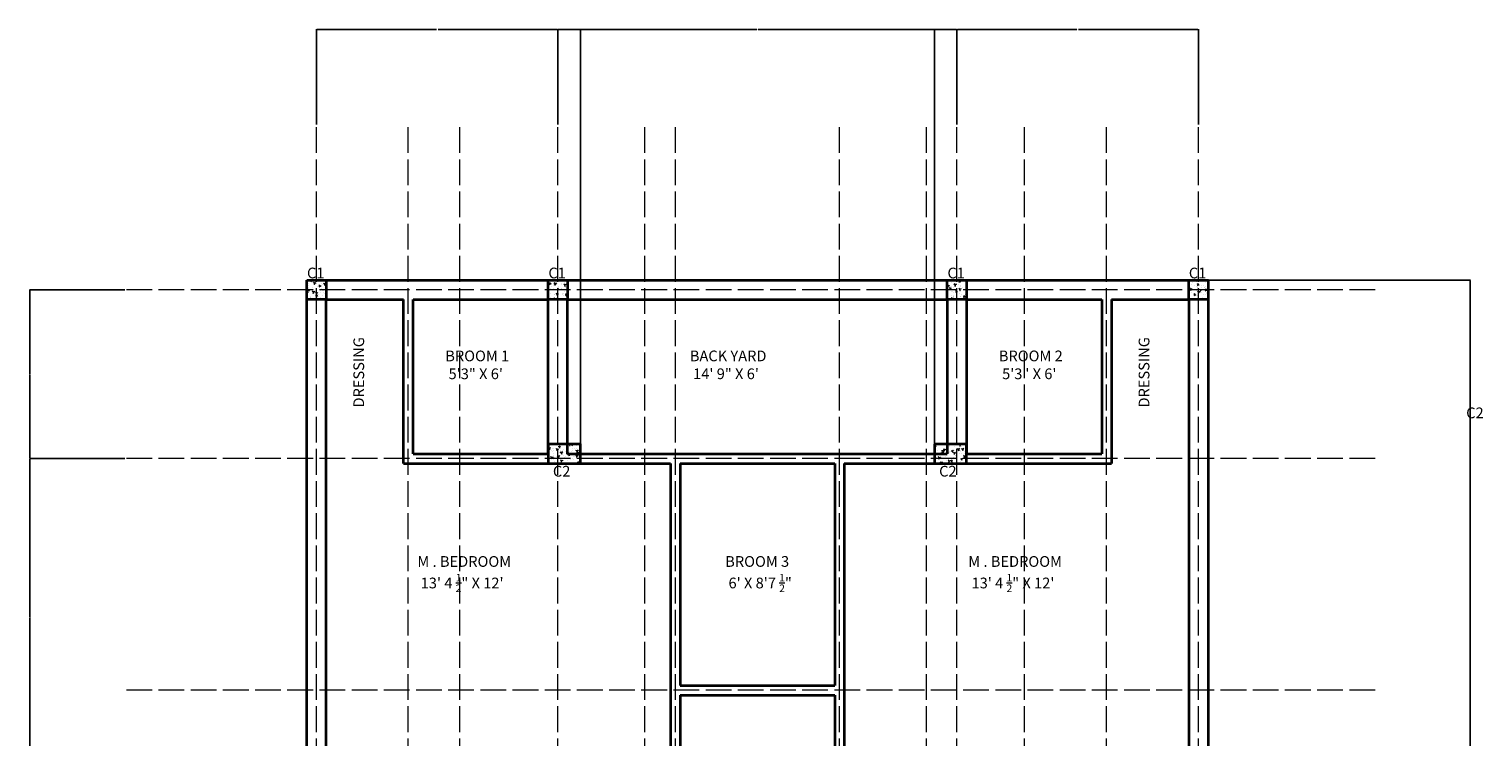
# Model space of a CAD drawing. Units: inches. Extents: x 1159 to 4240, y 1112 to 2085.
# Tile 12 of 13: x 2561 to 3239, y 1755 to 2085. Entities that reach past the tile are written whole.
import ezdxf

# ---------------------------------------------------------------- set-up
doc = ezdxf.new("R2010")
doc.units = ezdxf.units.IN
doc.linetypes.add('ACAD_ISO02W100', pattern=[15, 12, -3])
for name, color, linetype, lineweight in [('A-ANNO-DIMS', 2, 'Continuous', 18), ('A-AREA-IDEN', 30, 'Continuous', 18), ('A-GRID', 8, 'ACAD_ISO02W100', 13), ('COLUMN', 120, 'Continuous', 35), ('column no', 210, 'Continuous', 18), ('WALL', 7, 'Continuous', 35)]:
    doc.layers.add(name, color=color, linetype=linetype, lineweight=lineweight)
doc.styles.get("Standard").update_dxf_attribs({"font": 'arial.ttf'})
doc.dimstyles.get("Standard").update_dxf_attribs({"dimtxt": 0.18, "dimasz": 0.18, "dimexe": 0.18, "dimexo": 0.0625, "dimgap": 0.09, "dimtad": 0, "dimtih": 1, "dimtoh": 1, "dimdec": 4, "dimzin": 0, "dimdsep": 46, "dimtxsty": 'Standard', "dimcen": 0.09, "dimadec": 0, "dimazin": 0, "dimtfac": 1, "dimtdec": 4, "dimtofl": 0, "dimtmove": 0, "dimatfit": 3, "dimfxl": 1, "dimtolj": 1, "dimtzin": 0, "dimarcsym": 0})

# ---------------------------------------------------------------- blocks, each defined once
blk = doc.blocks.new('column')
at = {"layer": 'COLUMN'}
h = blk.add_hatch(dxfattribs=at)
h.set_pattern_fill('AR-CONC', color=256, scale=0.025)
h.set_pattern_definition([(50, (-3308.5408, -1592.3894), (4.5546167, -0.398477), [0.47625, -5.23875]), (355, (-3308.541, -1592.3894), (-0.8810855, 4.776421), [0.381, -4.1910146]), (100.45144, (-3308.1612, -1592.4226), (3.673531, 4.377944), [0.40475, -4.452256]), (46.1842, (-3308.541, -1591.1194), (6.776976, -1.051058), [0.714375, -7.858125]), (96.63556, (-3307.976, -1591.207), (5.935103, 6.185653), [0.607126, -6.67839]), (351.18415, (-3308.541, -1591.1194), (5.935103, 6.185653), [0.571499, -6.286493]), (21, (-3307.9058, -1591.437), (3.7903598, -2.55663), [0.47625, -5.23875]), (326, (-3307.906, -1591.437), (1.545051, 4.604699), [0.381, -4.191]), (71.45144, (-3307.59, -1591.65), (5.3354105, 2.048069), [0.40475, -4.4522484]), (37.5, (-3308.5408, -1592.3894), (0.0772151, 2.113876), [0, -4.1402, 0, -4.2545, 0, -4.206875]), (7.5, (-3308.5408, -1592.3894), (1.6704916, 2.5045144), [0, -2.4257, 0, -4.04495, 0, -1.603375]), (327.5, (-3309.9568, -1592.3894), (3.3897649, -0.1432186), [0, -1.5875, 0, -4.953, 0, -6.57225]), (317.5, (-3310.5918, -1592.3894), (3.7032295, 0.6356623), [0, -2.06375, 0, -3.2893, 0, -4.66725])])
h.paths.add_polyline_path([(0, 9), (0, 0), (9, 0), (9, 9)])
blk.add_lwpolyline([(0, 9), (9, 9), (9, 0), (0, 0)], close=True, dxfattribs=at)
blk = doc.blocks.new('colum 1')
at = {"layer": 'COLUMN'}
h = blk.add_hatch(dxfattribs=at)
h.set_pattern_fill('AR-CONC', color=256, scale=0.025)
h.set_pattern_definition([(50, (-3344.692, -1599.4877), (4.5546167, -0.398477), [0.47625, -5.23875]), (355, (-3344.692, -1599.4877), (-0.8810855, 4.776421), [0.381, -4.1910146]), (100.45144, (-3344.3125, -1599.521), (3.673531, 4.377944), [0.40475, -4.452256]), (46.1842, (-3344.692, -1598.218), (6.776976, -1.051058), [0.714375, -7.858125]), (96.63556, (-3344.127, -1598.305), (5.935103, 6.185653), [0.607126, -6.67839]), (351.18415, (-3344.692, -1598.218), (5.935103, 6.185653), [0.571499, -6.286493]), (21, (-3344.057, -1598.5352), (3.7903598, -2.55663), [0.47625, -5.23875]), (326, (-3344.057, -1598.5352), (1.545051, 4.604699), [0.381, -4.191]), (71.45144, (-3343.741, -1598.7483), (5.3354105, 2.048069), [0.40475, -4.4522484]), (37.5, (-3344.692, -1599.4877), (0.0772151, 2.113876), [0, -4.1402, 0, -4.2545, 0, -4.206875]), (7.5, (-3344.692, -1599.4877), (1.6704916, 2.5045144), [0, -2.4257, 0, -4.04495, 0, -1.603375]), (327.5, (-3346.1081, -1599.4877), (3.3897649, -0.1432186), [0, -1.5875, 0, -4.953, 0, -6.57225]), (317.5, (-3346.743, -1599.4877), (3.7032295, 0.6356623), [0, -2.06375, 0, -3.2893, 0, -4.66725])])
h.paths.add_polyline_path([(9, 15), (0, 15), (0, 0), (9, 0)])
blk.add_lwpolyline([(0, 0), (9, 0), (9, 15), (0, 15)], close=True, dxfattribs=at)
blk = doc.blocks.new('HOUSE-35x60-WALL-LAYOUT')
for p, q in [((0, 0), (0, 720)), ((0, 720), (420, 720)), ((420, 720), (420, 297)), ((9, 711), (45, 711)), ((9, 634.5), (9, 711)), ((45, 634.5), (45, 711)), ((49.5, 639), (49.5, 711)), ((49.5, 711), (112.5, 711)), ((112.5, 639), (112.5, 711)), ((121.5, 639), (121.5, 711)), ((121.5, 711), (298.5, 711)), ((298.5, 711), (298.5, 639)), ((307.5, 711), (307.5, 639)), ((307.5, 711), (370.5, 711)), ((370.5, 711), (370.5, 639)), ((375, 711), (375, 634.5)), ((375, 711), (411, 711)), ((411, 711), (411, 634.5)), ((49.5, 639), (112.5, 639)), ((121.5, 639), (298.5, 639)), ((307.5, 639), (370.5, 639)), ((9, 490.5), (9, 634.5)), ((45, 634.5), (169.5, 634.5)), ((169.5, 634.5), (169.5, 490.5)), ((174, 634.5), (174, 531)), ((174, 634.5), (246, 634.5)), ((246, 634.5), (246, 531)), ((250.5, 634.5), (250.5, 490.5)), ((250.5, 634.5), (375, 634.5)), ((411, 634.5), (411, 490.5)), ((174, 531), (246, 531)), ((174, 526.5), (246, 526.5)), ((174, 526.5), (174, 486)), ((246, 526.5), (246, 486)), ((9, 490.5), (169.5, 490.5)), ((250.5, 490.5), (411, 490.5)), ((9, 486), (174, 486)), ((9, 306), (9, 486)), ((246, 486), (286.5, 486)), ((286.5, 486), (286.5, 421.5)), ((291, 486), (291, 426)), ((291, 486), (411, 486)), ((411, 486), (411, 426)), ((291, 421.5), (286.5, 421.5)), ((291, 426), (411, 426)), ((291, 421.5), (411, 421.5)), ((411, 421.5), (411, 306)), ((291, 361.5), (286.5, 361.5)), ((286.5, 361.5), (286.5, 297)), ((291, 361.5), (291, 306)), ((9, 306), (157.5, 306)), ((157.5, 190.5), (157.5, 306)), ((291, 306), (411, 306)), ((9, 297), (153, 297)), ((9, 190.5), (9, 297)), ((153, 190.5), (153, 297)), ((286.5, 297), (420, 297)), ((330, 297), (330, 123)), ((339, 297), (339, 114)), ((153, 190.5), (9, 190.5)), ((157.5, 123), (157.5, 190.5)), ((9, 66), (9, 186)), ((153, 186), (9, 186)), ((153, 66), (153, 186)), ((330, 123), (157.5, 123)), ((162, 57), (162, 114)), ((339, 114), (162, 114)), ((153, 66), (9, 66)), ((9, 9), (9, 57)), ((69, 57), (9, 57)), ((69, 9), (69, 57)), ((162, 57), (73.5, 57)), ((73.5, 0), (73.5, 57)), ((69, 9), (9, 9)), ((0, 0), (73.5, 0))]:
    blk.add_line(p, q)
blk = doc.blocks.new('HOUSE-35x60-SETTING-OUT-GRID')
for p, q in [((89.32, 0), (89.32, 883.25)), ((132.07, 0), (132.07, 883.25)), ((156.07, 0), (156.07, 883.25)), ((201.82, 0), (201.82, 883.25)), ((242.32, 0), (242.32, 883.25)), ((256.57, 0), (256.57, 883.25)), ((333.07, 0), (333.07, 883.25)), ((373.57, 0), (373.57, 883.25)), ((387.82, 0), (387.82, 883.25)), ((419.32, 0), (419.32, 883.25)), ((457.57, 0), (457.57, 883.25)), ((500.32, 0), (500.32, 883.25)), ((582.7, 806.25), (0, 806.25)), ((582.7, 727.5), (0, 727.5)), ((582.7, 619.5), (0, 619.5)), ((582.7, 579), (0, 579)), ((582.7, 514.5), (0, 514.5)), ((582.7, 392.25), (0, 392.25)), ((582.7, 279), (0, 279)), ((582.7, 209.25), (0, 209.25)), ((582.7, 152.25), (0, 152.25)), ((582.7, 95.25), (0, 95.25))]:
    blk.add_line(p, q)
blk = doc.blocks.new('*D25')
at = {"layer": 'A-ANNO-DIMS', "color": 0, "lineweight": -2, "transparency": 16777216}
for p, q in [((3110.55, 1967.7), (3232.9, 1967.7)), ((3232.72, 1967.52), (3232.72, 1607.88)), ((3232.72, 1247.88), (3232.72, 1607.52)), ((3110.55, 1247.7), (3232.9, 1247.7))]:
    blk.add_line(p, q, dxfattribs=at)
at = {"layer": 'A-ANNO-DIMS', "color": 0, "lineweight": 100, "transparency": 16777216}
for points in [[(3232.69, 1967.52), (3232.75, 1967.52), (3232.72, 1967.7)], [(3232.69, 1247.88), (3232.75, 1247.88), (3232.72, 1247.7)]]:
    blk.add_solid(points, dxfattribs=at)
at = {"layer": 'Defpoints', "color": 0, "lineweight": 100, "transparency": 16777216}
for p in [(3110.48, 1967.7), (3232.72, 1967.7), (3110.48, 1247.7)]:
    blk.add_point(p, dxfattribs=at)
at = {"layer": 'A-ANNO-DIMS', "color": 0, "transparency": 16777216, "insert": (3232.72, 1607.7), "char_height": 0.18, "attachment_point": 5}
blk.add_mtext('\\A1;720', dxfattribs=at)
blk = doc.blocks.new('*D46')
at = {"layer": 'A-ANNO-DIMS', "color": 0, "lineweight": -2, "transparency": 16777216}
for p, q in [((2694.98, 2040.27), (2694.98, 2084.73)), ((2695.16, 2084.55), (2750.85, 2084.55)), ((2807.3, 2084.55), (2751.62, 2084.55)), ((2807.48, 2040.27), (2807.48, 2084.73))]:
    blk.add_line(p, q, dxfattribs=at)
at = {"layer": 'A-ANNO-DIMS', "color": 0, "lineweight": 100, "transparency": 16777216}
for points in [[(2695.16, 2084.58), (2695.16, 2084.52), (2694.98, 2084.55)], [(2807.3, 2084.58), (2807.3, 2084.52), (2807.48, 2084.55)]]:
    blk.add_solid(points, dxfattribs=at)
at = {"layer": 'Defpoints', "color": 0, "lineweight": 100, "transparency": 16777216}
for p in [(2807.48, 2084.55), (2694.98, 2040.2), (2807.48, 2040.2)]:
    blk.add_point(p, dxfattribs=at)
at = {"layer": 'A-ANNO-DIMS', "color": 0, "transparency": 16777216, "insert": (2751.23, 2084.55), "char_height": 0.18, "attachment_point": 5}
blk.add_mtext('\\A1;112.5', dxfattribs=at)
blk = doc.blocks.new('*D47')
at = {"layer": 'A-ANNO-DIMS', "color": 0, "lineweight": -2, "transparency": 16777216}
for p, q in [((2807.48, 2040.27), (2807.48, 2084.73)), ((2807.66, 2084.55), (2900.2, 2084.55)), ((2993.3, 2084.55), (2900.76, 2084.55)), ((2993.48, 2040.27), (2993.48, 2084.73))]:
    blk.add_line(p, q, dxfattribs=at)
at = {"layer": 'A-ANNO-DIMS', "color": 0, "lineweight": 100, "transparency": 16777216}
for points in [[(2807.66, 2084.58), (2807.66, 2084.52), (2807.48, 2084.55)], [(2993.3, 2084.58), (2993.3, 2084.52), (2993.48, 2084.55)]]:
    blk.add_solid(points, dxfattribs=at)
at = {"layer": 'Defpoints', "color": 0, "lineweight": 100, "transparency": 16777216}
for p in [(2993.48, 2084.55), (2807.48, 2040.2), (2993.48, 2040.2)]:
    blk.add_point(p, dxfattribs=at)
at = {"layer": 'A-ANNO-DIMS', "color": 0, "transparency": 16777216, "insert": (2900.48, 2084.55), "char_height": 0.18, "attachment_point": 5}
blk.add_mtext('\\A1;186', dxfattribs=at)
blk = doc.blocks.new('*D48')
at = {"layer": 'A-ANNO-DIMS', "color": 0, "lineweight": -2, "transparency": 16777216}
for p, q in [((2993.48, 2040.27), (2993.48, 2084.73)), ((2993.66, 2084.55), (3049.35, 2084.55)), ((3105.8, 2084.55), (3050.12, 2084.55)), ((3105.98, 2040.27), (3105.98, 2084.73))]:
    blk.add_line(p, q, dxfattribs=at)
at = {"layer": 'A-ANNO-DIMS', "color": 0, "lineweight": 100, "transparency": 16777216}
for points in [[(2993.66, 2084.58), (2993.66, 2084.52), (2993.48, 2084.55)], [(3105.8, 2084.58), (3105.8, 2084.52), (3105.98, 2084.55)]]:
    blk.add_solid(points, dxfattribs=at)
at = {"layer": 'Defpoints', "color": 0, "lineweight": 100, "transparency": 16777216}
for p in [(3105.98, 2084.55), (2993.48, 2040.2), (3105.98, 2040.2)]:
    blk.add_point(p, dxfattribs=at)
at = {"layer": 'A-ANNO-DIMS', "color": 0, "transparency": 16777216, "insert": (3049.73, 2084.55), "char_height": 0.18, "attachment_point": 5}
blk.add_mtext('\\A1;112.5', dxfattribs=at)
blk = doc.blocks.new('*D50')
at = {"layer": 'A-ANNO-DIMS', "color": 0, "lineweight": -2, "transparency": 16777216}
for p, q in [((2605.61, 1884.45), (2561.14, 1884.45)), ((2561.32, 1884.27), (2561.32, 1810.38)), ((2561.32, 1736.13), (2561.32, 1810.02)), ((2605.61, 1735.95), (2561.14, 1735.95))]:
    blk.add_line(p, q, dxfattribs=at)
at = {"layer": 'A-ANNO-DIMS', "color": 0, "lineweight": 100, "transparency": 16777216}
for points in [[(2561.29, 1884.27), (2561.35, 1884.27), (2561.32, 1884.45)], [(2561.29, 1736.13), (2561.35, 1736.13), (2561.32, 1735.95)]]:
    blk.add_solid(points, dxfattribs=at)
at = {"layer": 'Defpoints', "color": 0, "lineweight": 100, "transparency": 16777216}
for p in [(2561.32, 1884.45), (2605.67, 1884.45), (2605.67, 1735.95)]:
    blk.add_point(p, dxfattribs=at)
at = {"layer": 'A-ANNO-DIMS', "color": 0, "transparency": 16777216, "insert": (2561.32, 1810.2), "char_height": 0.18, "attachment_point": 5}
blk.add_mtext('\\A1;148.5', dxfattribs=at)
blk = doc.blocks.new('*D51')
at = {"layer": 'A-ANNO-DIMS', "color": 0, "lineweight": -2, "transparency": 16777216}
for p, q in [((2605.61, 1963.2), (2561.14, 1963.2)), ((2561.32, 1963.02), (2561.32, 1924.01)), ((2561.32, 1884.63), (2561.32, 1923.65)), ((2605.61, 1884.45), (2561.14, 1884.45))]:
    blk.add_line(p, q, dxfattribs=at)
at = {"layer": 'A-ANNO-DIMS', "color": 0, "lineweight": 100, "transparency": 16777216}
for points in [[(2561.29, 1963.02), (2561.35, 1963.02), (2561.32, 1963.2)], [(2561.29, 1884.63), (2561.35, 1884.63), (2561.32, 1884.45)]]:
    blk.add_solid(points, dxfattribs=at)
at = {"layer": 'Defpoints', "color": 0, "lineweight": 100, "transparency": 16777216}
for p in [(2561.32, 1963.2), (2605.67, 1963.2), (2605.67, 1884.45)]:
    blk.add_point(p, dxfattribs=at)
at = {"layer": 'A-ANNO-DIMS', "color": 0, "transparency": 16777216, "insert": (2561.32, 1923.83), "char_height": 0.18, "attachment_point": 5}
blk.add_mtext('\\A1;78.75', dxfattribs=at)
blk = doc.blocks.new('*D52')
at = {"layer": 'A-ANNO-DIMS', "color": 0, "lineweight": -2, "transparency": 16777216}
for p, q in [((2817.98, 1891.26), (2817.98, 2084.73)), ((2818.16, 2084.55), (2900.2, 2084.55)), ((2982.8, 2084.55), (2900.76, 2084.55)), ((2982.98, 1891.26), (2982.98, 2084.73))]:
    blk.add_line(p, q, dxfattribs=at)
at = {"layer": 'A-ANNO-DIMS', "color": 0, "lineweight": 100, "transparency": 16777216}
for points in [[(2818.16, 2084.58), (2818.16, 2084.52), (2817.98, 2084.55)], [(2982.8, 2084.58), (2982.8, 2084.52), (2982.98, 2084.55)]]:
    blk.add_solid(points, dxfattribs=at)
at = {"layer": 'Defpoints', "color": 0, "lineweight": 100, "transparency": 16777216}
for p in [(2982.98, 2084.55), (2817.98, 1891.2), (2982.98, 1891.2)]:
    blk.add_point(p, dxfattribs=at)
at = {"layer": 'A-ANNO-DIMS', "color": 0, "transparency": 16777216, "insert": (2900.48, 2084.55), "char_height": 0.18, "attachment_point": 5}
blk.add_mtext('\\A1;165', dxfattribs=at)

msp = doc.modelspace()

# ---------------------------------------------------------------- block references
at = {"layer": 'A-GRID'}
msp.add_blockref('HOUSE-35x60-SETTING-OUT-GRID', (2605.668, 1156.954), dxfattribs=at)
at = {"layer": 'COLUMN'}
for p in [(2690.484, 1958.702), (2802.984, 1958.702), (2988.984, 1958.702), (3101.484, 1958.702)]:
    msp.add_blockref('column', p, dxfattribs=at)
at = {"layer": 'COLUMN', "rotation": 270}
for p in [(2802.984, 1891.202), (2982.984, 1891.202)]:
    msp.add_blockref('colum 1', p, dxfattribs=at)
at = {"layer": 'WALL'}
msp.add_blockref('HOUSE-35x60-WALL-LAYOUT', (2690.484, 1247.702), dxfattribs=at)

# ---------------------------------------------------------------- texts
at = {"layer": 'A-AREA-IDEN', "char_height": 5, "attachment_point": 1, "rotation": 90}
for insert in [(2712.173, 1908.276), (3078.173, 1908.276)]:
    msp.add_mtext_dynamic_manual_height_columns('\\A1;DRESSING', width=140.18614, gutter_width=12.5, heights=[0], dxfattribs=dict(at, insert=insert))
at = {"layer": 'A-AREA-IDEN', "char_height": 5, "attachment_point": 1}
for s, insert in [('\\A1;BROOM 1\\P 5\'3" X 6\'', (2754.996, 1934.831)), ('\\A1;BACK YARD\\P 14\' 9" X 6\'', (2868.983, 1934.831)), ('\\A1;BROOM 2\\P 5\'3" X 6\'', (3012.996, 1934.831)), ('\\A1;M . BEDROOM\\P 13\' 4 {\\H0.7x;\\S1/2;}" X 12\'', (2742.008, 1838.992)), ('\\A1;BROOM 3\\P 6\' X 8\'7 {\\H0.7x;\\S1/2;}"', (2885.474, 1838.992)), ('\\A1;M . BEDROOM\\P 13\' 4 {\\H0.7x;\\S1/2;}" X 12\'', (2998.748, 1838.992))]:
    msp.add_mtext_dynamic_manual_height_columns(s, width=140.18614, gutter_width=12.5, heights=[0], dxfattribs=dict(at, insert=insert))
at = {"layer": 'column no', "char_height": 5, "attachment_point": 1}
for s, insert in [('\\A1;C1', (2690.549, 1973.493)), ('\\A1;C1', (2803.049, 1973.493)), ('\\A1;C1', (2989.049, 1973.493)), ('\\A1;C1', (3101.549, 1973.493)), ('\\A1;C2', (3230.822, 1908.276)), ('\\A1;C2', (2805.162, 1881.077)), ('\\A1;C2', (2985.163, 1881.077))]:
    msp.add_mtext_dynamic_manual_height_columns(s, width=140.18614, gutter_width=12.5, heights=[0], dxfattribs=dict(at, insert=insert))

# ---------------------------------------------------------------- dimensions: what is measured, and where the dimension line sits
at = {"layer": 'A-ANNO-DIMS'}
for base, p1, p2, override, picture, middle in [((2807.484, 2084.554), (2694.984, 2040.204), (2807.484, 2040.204), {"dimdec": 1, "dimlfac": 1, "dimrnd": 0, "dimzin": 0, "dimdsep": 46, "dimlunit": 2}, '*D46', (2751.234, 2084.554)), ((2993.484, 2084.554), (2807.484, 2040.204), (2993.484, 2040.204), {"dimdec": 0, "dimlfac": 1, "dimrnd": 0, "dimzin": 0, "dimdsep": 46, "dimlunit": 2}, '*D47', (2900.484, 2084.554)), ((2982.984, 2084.554), (2817.984, 1891.202), (2982.984, 1891.202), {"dimdec": 0, "dimlfac": 1, "dimrnd": 0, "dimzin": 0, "dimdsep": 46, "dimlunit": 2}, '*D52', (2900.484, 2084.554)), ((3105.984, 2084.554), (2993.484, 2040.204), (3105.984, 2040.204), {"dimdec": 1, "dimlfac": 1, "dimrnd": 0, "dimzin": 0, "dimdsep": 46, "dimlunit": 2}, '*D48', (3049.734, 2084.554))]:
    dim = msp.add_linear_dim(base=base, p1=p1, p2=p2, dimstyle='Standard', override=override, dxfattribs=at)
    dim.commit()
    dim.dimension.update_dxf_attribs({"geometry": picture, "text_midpoint": middle})
for base, p1, p2, override, picture, middle in [((3232.722, 1967.702), (3110.484, 1247.702), (3110.484, 1967.702), {"dimdec": 0, "dimlfac": 1, "dimrnd": 0, "dimzin": 0, "dimdsep": 46, "dimlunit": 2}, '*D25', (3232.722, 1607.702)), ((2561.318, 1963.202), (2605.668, 1884.452), (2605.668, 1963.202), {"dimdec": 2, "dimlfac": 1, "dimrnd": 0, "dimzin": 0, "dimdsep": 46, "dimlunit": 2}, '*D51', (2561.318, 1923.827)), ((2561.318, 1884.452), (2605.668, 1735.952), (2605.668, 1884.452), {"dimdec": 1, "dimlfac": 1, "dimrnd": 0, "dimzin": 0, "dimdsep": 46, "dimlunit": 2}, '*D50', (2561.318, 1810.202))]:
    dim = msp.add_linear_dim(base=base, p1=p1, p2=p2, angle=90, dimstyle='Standard', override=override, dxfattribs=at)
    dim.commit()
    dim.dimension.update_dxf_attribs({"geometry": picture, "text_midpoint": middle})

doc.saveas('drawing.dxf')
